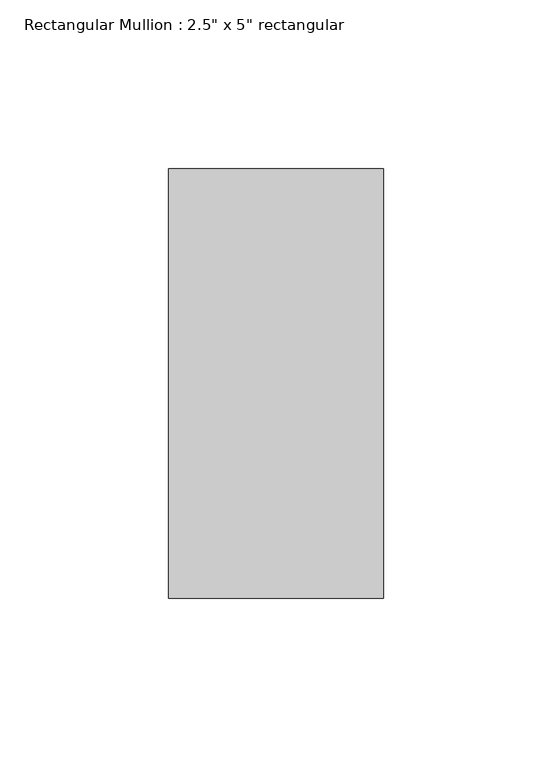
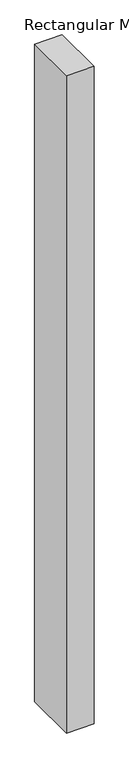
"""IFC4 building model written with IfcOpenShell, lengths in millimetres: member geometry."""

from ifc_helpers import new_model, si_unit, frame, origin, place, context, project, spatial, polyline, outline, extrude, source, transform, mapped, element, save


def member_de9b0c97(model_context):
    return source(origin(), model_context, "Body", "SweptSolid", [
        extrude(outline(polyline([(0.0, 63.5), (0.0, -63.5), (-63.5, -63.5), (-63.5, 63.5), (0.0, 63.5)])), frame((0.0, 0.0, -1606.2683749), z_axis=(0.0, 0.0, 1.0), x_axis=(1.0, 0.0, 0.0)), (0.0, 0.0, 1.0), 1606.2683749),
    ])


if __name__ == "__main__":
    model = new_model("IFC4")
    model_context = context("Model", 3, world=origin())
    ifc_project = project(units=[si_unit("LENGTHUNIT", "METRE", prefix="MILLI")], contexts=[model_context])
    site = spatial("IfcSite", under=ifc_project)
    building = spatial("IfcBuilding", under=site)
    placement = place(None, origin())
    member_shape = member_de9b0c97(model_context)
    element("IfcMember", 1, ObjectType="Rectangular Mullion : 2.5\" x 5\" rectangular", at=placement, inside=building, context=model_context, shape_type="MappedRepresentation", body=[
        mapped(member_shape, transform((0.0, 0.0, 0.0), x_axis=(1.0, 0.0, 0.0), y_axis=(0.0, 1.0, 0.0), z_axis=(0.0, 0.0, 1.0))),
    ])
    save(model, "model.ifc")

# Revit data of these elements
# Type "Rectangular Mullion : 2.5\" x 5\" rectangular"
#   built-in parameter 1007304 = 0.416667 (stored number, unit not read)
#   built-in parameter 1007301 = 0.104167 (stored number, unit not read)
#   built-in parameter 1007300 = 0.104167 (stored number, unit not read)
# Element 1 (IfcMember, "Rectangular Mullion : 2.5\" x 5\" rectangular")
#   Materials on its faces: "Aluminum"
# Materials
#   "Aluminum": class "Metal", colour RGB 247 247 247, transparency 0, Description = "Aluminum 6061", Cost = 0
